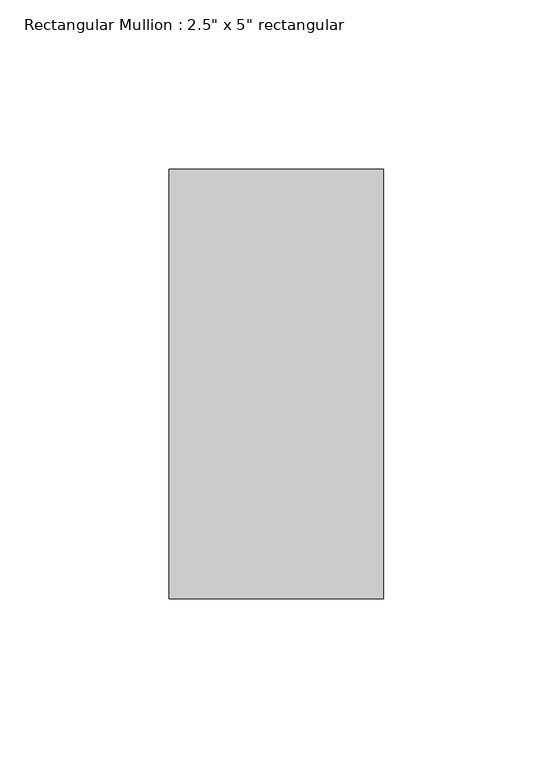
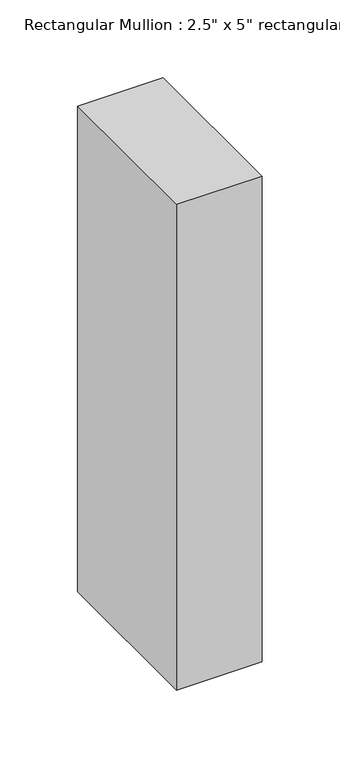
"""IFC4 building model written with IfcOpenShell, lengths in millimetres: member geometry."""

from ifc_helpers import new_model, si_unit, frame, origin, place, context, project, spatial, polyline, outline, extrude, source, transform, mapped, element, save


def member_03a502dc(model_context):
    return source(origin(), model_context, "Body", "SweptSolid", [
        extrude(outline(polyline([(31.75, 63.5), (31.75, -63.5), (-31.75, -63.5), (-31.75, 63.5), (31.75, 63.5)])), frame((0.0, 0.0, -381.0), z_axis=(0.0, 0.0, 1.0), x_axis=(1.0, 0.0, 0.0)), (0.0, 0.0, 1.0), 381.0),
    ])


if __name__ == "__main__":
    model = new_model("IFC4")
    model_context = context("Model", 3, world=origin())
    ifc_project = project(units=[si_unit("LENGTHUNIT", "METRE", prefix="MILLI")], contexts=[model_context])
    site = spatial("IfcSite", under=ifc_project)
    building = spatial("IfcBuilding", under=site)
    placement = place(None, origin())
    member_shape = member_03a502dc(model_context)
    element("IfcMember", 1, ObjectType="Rectangular Mullion : 2.5\" x 5\" rectangular", at=placement, inside=building, context=model_context, shape_type="MappedRepresentation", body=[
        mapped(member_shape, transform((0.0, 0.0, 0.0), x_axis=(1.0, 0.0, 0.0), y_axis=(0.0, 1.0, 0.0), z_axis=(0.0, 0.0, 1.0))),
    ])
    save(model, "model.ifc")

# Revit data of these elements
# Type "Rectangular Mullion : 2.5\" x 5\" rectangular"
#   built-in parameter 1007304 = 0.416667 (stored number, unit not read)
#   built-in parameter 1007301 = 0.104167 (stored number, unit not read)
#   built-in parameter 1007300 = 0.104167 (stored number, unit not read)
# Element 1 (IfcMember, "Rectangular Mullion : 2.5\" x 5\" rectangular")
#   Materials on its faces: "door colour"
# Materials
#   "door colour": class "Generic", colour RGB 120 120 120, transparency 0, Cost = 0
